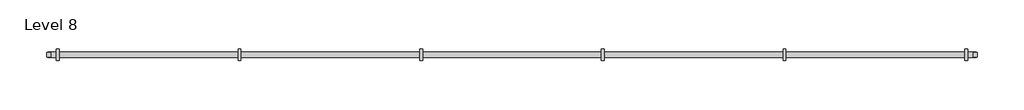
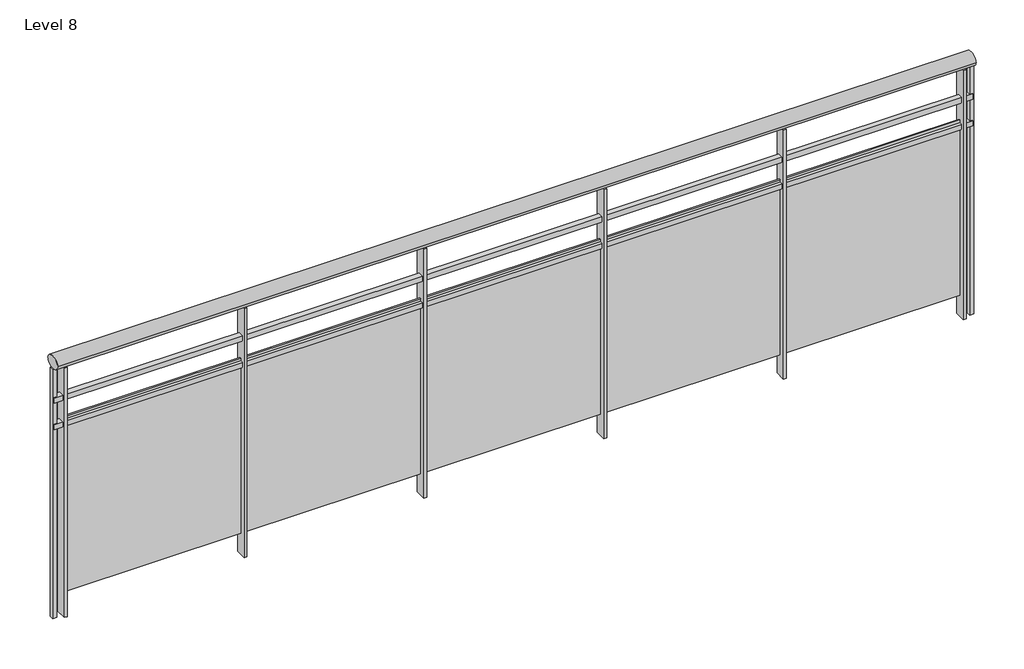
# One storey: 2 railings.
"""IFC4 building model written with IfcOpenShell, lengths in millimetres."""

from ifc_helpers import new_model, si_unit, point, frame, origin, place, context, project, spatial, polyline, ellipse_curve, trimmed, outline, extrude, element, save
from ifc_brep_helpers import plane_surface, extruded_surface, advanced_brep

model = new_model("IFC4")

# Units and contexts
model_context = context("Model", 3, world=origin())
ifc_project = project(units=[si_unit("LENGTHUNIT", "METRE", prefix="MILLI")], contexts=[model_context])

# Site, building, storey
site = spatial("IfcSite", under=ifc_project)
building = spatial("IfcBuilding", under=site)
storey = spatial("IfcBuildingStorey", under=building, Name="Level 8", Elevation=22402.8)

# Railings
placement = place(None, origin())
element("IfcRailing", 1, ObjectType="Glass Panel - Bottom Fill", at=placement, inside=storey, context=model_context, shape_type="SolidModel", body=[
    advanced_brep(
    [(-5729.1673724, -5829.5544725, 23622.0), (-5729.1673724, -5905.7544725, 23622.0), (-1576.8982041, -5829.5544725, 23622.0), (-1576.8982041, -5905.7544725, 23622.0)],
    [
        (0, 1, ellipse_curve(frame((-5729.1673724, -5867.6544725, 23622.0), z_axis=(-1.0, 0.0, 0.0), x_axis=(0.0, -1.0, 0.0)), 38.1, 28.575)),
        (1, 0, ellipse_curve(frame((-5729.1673724, -5867.6544725, 23622.0), z_axis=(-1.0, 0.0, 0.0), x_axis=(0.0, -1.0, 0.0)), 38.1, 28.575)),
        (2, 3, ellipse_curve(frame((-1576.8982041, -5867.6544725, 23622.0), z_axis=(1.0, 0.0, 0.0), x_axis=(0.0, -1.0, 0.0)), 38.1, 28.575)),
        (3, 2, ellipse_curve(frame((-1576.8982041, -5867.6544725, 23622.0), z_axis=(1.0, 0.0, 0.0), x_axis=(0.0, -1.0, 0.0)), 38.1, 28.575)),
        (0, 2),
        (3, 1),
    ],
    [
        plane_surface(frame((-5729.1673724, -5867.6544725, 23622.0), z_axis=(-1.0, 0.0, 0.0), x_axis=(0.0, 1.0, 0.0))),
        plane_surface(frame((-1576.8982041, -5867.6544725, 23622.0), z_axis=(1.0, 0.0, 0.0), x_axis=(0.0, 1.0, 0.0))),
        extruded_surface(trimmed(ellipse_curve(frame((-1576.8982041, -5867.6544725, 23622.0), z_axis=(-1.0, 0.0, 0.0), x_axis=(0.0, -1.0, 0.0)), 38.1, 28.575), [point((-1576.8982041, -5829.5544725, 23622.0))], [point((-1576.8982041, -5905.7544725, 23622.0))], True, "CARTESIAN"), (-4152.2691683, 0.0, 0.0), 4152.2691683),
        extruded_surface(trimmed(ellipse_curve(frame((-1576.8982041, -5867.6544725, 23622.0), z_axis=(-1.0, 0.0, 0.0), x_axis=(0.0, -1.0, 0.0)), 38.1, 28.575), [point((-1576.8982041, -5905.7544725, 23622.0))], [point((-1576.8982041, -5829.5544725, 23622.0))], True, "CARTESIAN"), (-4152.2691683, 0.0, 0.0), 4152.2691683),
    ],
    [
        (0, [[1, 2]]),
        (1, [[3, 4]]),
        (2, [[-1, 5, -4, 6]]),
        (3, [[-2, -6, -3, -5]]),
    ],
),
    extrude(outline(polyline([(-5729.1673724, -5880.3544725), (-5729.1673724, -5854.9544725), (-1576.8982041, -5854.9544725), (-1576.8982041, -5880.3544725), (-5729.1673724, -5880.3544725)])), frame((0.0, 0.0, 23431.5), z_axis=(0.0, 0.0, 1.0), x_axis=(1.0, 0.0, 0.0)), (0.0, 0.0, 1.0), 25.4),
    extrude(outline(polyline([(-5729.1673724, -5880.3544725), (-5729.1673724, -5854.9544725), (-1576.8982041, -5854.9544725), (-1576.8982041, -5880.3544725), (-5729.1673724, -5880.3544725)])), frame((0.0, 0.0, 23304.5), z_axis=(0.0, 0.0, 1.0), x_axis=(1.0, 0.0, 0.0)), (0.0, 0.0, 1.0), 25.4),
    extrude(outline(polyline([(-1627.3827882, -5893.0544725), (-1627.3827882, -5842.2544725), (-1614.6827882, -5842.2544725), (-1614.6827882, -5893.0544725), (-1627.3827882, -5893.0544725)])), frame((0.0, 0.0, 22402.8), z_axis=(0.0, 0.0, 1.0), x_axis=(1.0, 0.0, 0.0)), (0.0, 0.0, 1.0), 1190.625),
    extrude(outline(polyline([(-2433.8327882, -5861.1193155), (-1621.0327882, -5861.1193155), (-1621.0327882, -5867.4693155), (-2433.8327882, -5867.4693155), (-2433.8327882, -5861.1193155)])), frame((0.0, 0.0, 22504.4), z_axis=(0.0, 0.0, 1.0), x_axis=(1.0, 0.0, 0.0)), (0.0, 0.0, 1.0), 838.2),
    extrude(outline(polyline([(-2440.1827882, -5893.0544725), (-2440.1827882, -5842.2544725), (-2427.4827882, -5842.2544725), (-2427.4827882, -5893.0544725), (-2440.1827882, -5893.0544725)])), frame((0.0, 0.0, 22402.8), z_axis=(0.0, 0.0, 1.0), x_axis=(1.0, 0.0, 0.0)), (0.0, 0.0, 1.0), 1190.625),
    extrude(outline(polyline([(-3246.6327882, -5861.1193155), (-2433.8327882, -5861.1193155), (-2433.8327882, -5867.4693155), (-3246.6327882, -5867.4693155), (-3246.6327882, -5861.1193155)])), frame((0.0, 0.0, 22504.4), z_axis=(0.0, 0.0, 1.0), x_axis=(1.0, 0.0, 0.0)), (0.0, 0.0, 1.0), 838.2),
    extrude(outline(polyline([(-3252.9827882, -5893.0544725), (-3252.9827882, -5842.2544725), (-3240.2827882, -5842.2544725), (-3240.2827882, -5893.0544725), (-3252.9827882, -5893.0544725)])), frame((0.0, 0.0, 22402.8), z_axis=(0.0, 0.0, 1.0), x_axis=(1.0, 0.0, 0.0)), (0.0, 0.0, 1.0), 1190.625),
    extrude(outline(polyline([(-4059.4327882, -5861.1193155), (-3246.6327882, -5861.1193155), (-3246.6327882, -5867.4693155), (-4059.4327882, -5867.4693155), (-4059.4327882, -5861.1193155)])), frame((0.0, 0.0, 22504.4), z_axis=(0.0, 0.0, 1.0), x_axis=(1.0, 0.0, 0.0)), (0.0, 0.0, 1.0), 838.2),
    extrude(outline(polyline([(-4065.7827882, -5893.0544725), (-4065.7827882, -5842.2544725), (-4053.0827882, -5842.2544725), (-4053.0827882, -5893.0544725), (-4065.7827882, -5893.0544725)])), frame((0.0, 0.0, 22402.8), z_axis=(0.0, 0.0, 1.0), x_axis=(1.0, 0.0, 0.0)), (0.0, 0.0, 1.0), 1190.625),
    extrude(outline(polyline([(-4872.2327882, -5861.1193155), (-4059.4327882, -5861.1193155), (-4059.4327882, -5867.4693155), (-4872.2327882, -5867.4693155), (-4872.2327882, -5861.1193155)])), frame((0.0, 0.0, 22504.4), z_axis=(0.0, 0.0, 1.0), x_axis=(1.0, 0.0, 0.0)), (0.0, 0.0, 1.0), 838.2),
    extrude(outline(polyline([(-4878.5827882, -5893.0544725), (-4878.5827882, -5842.2544725), (-4865.8827882, -5842.2544725), (-4865.8827882, -5893.0544725), (-4878.5827882, -5893.0544725)])), frame((0.0, 0.0, 22402.8), z_axis=(0.0, 0.0, 1.0), x_axis=(1.0, 0.0, 0.0)), (0.0, 0.0, 1.0), 1190.625),
    extrude(outline(polyline([(-5685.0327882, -5861.1193155), (-4872.2327882, -5861.1193155), (-4872.2327882, -5867.4693155), (-5685.0327882, -5867.4693155), (-5685.0327882, -5861.1193155)])), frame((0.0, 0.0, 22504.4), z_axis=(0.0, 0.0, 1.0), x_axis=(1.0, 0.0, 0.0)), (0.0, 0.0, 1.0), 838.2),
    extrude(outline(polyline([(-5691.3827882, -5893.0544725), (-5691.3827882, -5842.2544725), (-5678.6827882, -5842.2544725), (-5678.6827882, -5893.0544725), (-5691.3827882, -5893.0544725)])), frame((0.0, 0.0, 22402.8), z_axis=(0.0, 0.0, 1.0), x_axis=(1.0, 0.0, 0.0)), (0.0, 0.0, 1.0), 1190.625),
    extrude(outline(polyline([(-1589.5982041, -5877.1794725), (-1589.5982041, -5858.1294725), (-1570.5482041, -5858.1294725), (-1570.5482041, -5877.1794725), (-1589.5982041, -5877.1794725)])), frame((0.0, 0.0, 22402.8), z_axis=(0.0, 0.0, 1.0), x_axis=(1.0, 0.0, 0.0)), (0.0, 0.0, 1.0), 1190.625),
    extrude(outline(polyline([(-5735.5173724, -5877.1794725), (-5735.5173724, -5858.1294725), (-5716.4673724, -5858.1294725), (-5716.4673724, -5877.1794725), (-5735.5173724, -5877.1794725)])), frame((0.0, 0.0, 22402.8), z_axis=(0.0, 0.0, 1.0), x_axis=(1.0, 0.0, 0.0)), (0.0, 0.0, 1.0), 1190.625),
])
element("IfcRailing", 2, ObjectType="Glass Panel - Bottom Fill", at=placement, inside=storey, context=model_context, shape_type="SolidModel", body=[
    advanced_brep(
    [(-5729.1673724, -5829.5544725, 23622.0), (-5729.1673724, -5905.7544725, 23622.0), (-1576.8982041, -5829.5544725, 23622.0), (-1576.8982041, -5905.7544725, 23622.0)],
    [
        (0, 1, ellipse_curve(frame((-5729.1673724, -5867.6544725, 23622.0), z_axis=(-1.0, 0.0, 0.0), x_axis=(0.0, -1.0, 0.0)), 38.1, 28.575)),
        (1, 0, ellipse_curve(frame((-5729.1673724, -5867.6544725, 23622.0), z_axis=(-1.0, 0.0, 0.0), x_axis=(0.0, -1.0, 0.0)), 38.1, 28.575)),
        (2, 3, ellipse_curve(frame((-1576.8982041, -5867.6544725, 23622.0), z_axis=(1.0, 0.0, 0.0), x_axis=(0.0, -1.0, 0.0)), 38.1, 28.575)),
        (3, 2, ellipse_curve(frame((-1576.8982041, -5867.6544725, 23622.0), z_axis=(1.0, 0.0, 0.0), x_axis=(0.0, -1.0, 0.0)), 38.1, 28.575)),
        (0, 2),
        (3, 1),
    ],
    [
        plane_surface(frame((-5729.1673724, -5867.6544725, 23622.0), z_axis=(-1.0, 0.0, 0.0), x_axis=(0.0, 1.0, 0.0))),
        plane_surface(frame((-1576.8982041, -5867.6544725, 23622.0), z_axis=(1.0, 0.0, 0.0), x_axis=(0.0, 1.0, 0.0))),
        extruded_surface(trimmed(ellipse_curve(frame((-1576.8982041, -5867.6544725, 23622.0), z_axis=(-1.0, 0.0, 0.0), x_axis=(0.0, -1.0, 0.0)), 38.1, 28.575), [point((-1576.8982041, -5829.5544725, 23622.0))], [point((-1576.8982041, -5905.7544725, 23622.0))], True, "CARTESIAN"), (-4152.2691683, 0.0, 0.0), 4152.2691683),
        extruded_surface(trimmed(ellipse_curve(frame((-1576.8982041, -5867.6544725, 23622.0), z_axis=(-1.0, 0.0, 0.0), x_axis=(0.0, -1.0, 0.0)), 38.1, 28.575), [point((-1576.8982041, -5905.7544725, 23622.0))], [point((-1576.8982041, -5829.5544725, 23622.0))], True, "CARTESIAN"), (-4152.2691683, 0.0, 0.0), 4152.2691683),
    ],
    [
        (0, [[1, 2]]),
        (1, [[3, 4]]),
        (2, [[-1, 5, -4, 6]]),
        (3, [[-2, -6, -3, -5]]),
    ],
),
    extrude(outline(polyline([(-5729.1673724, -5880.3544725), (-5729.1673724, -5854.9544725), (-1576.8982041, -5854.9544725), (-1576.8982041, -5880.3544725), (-5729.1673724, -5880.3544725)])), frame((0.0, 0.0, 23431.5), z_axis=(0.0, 0.0, 1.0), x_axis=(1.0, 0.0, 0.0)), (0.0, 0.0, 1.0), 25.4),
    extrude(outline(polyline([(-5729.1673724, -5880.3544725), (-5729.1673724, -5854.9544725), (-1576.8982041, -5854.9544725), (-1576.8982041, -5880.3544725), (-5729.1673724, -5880.3544725)])), frame((0.0, 0.0, 23304.5), z_axis=(0.0, 0.0, 1.0), x_axis=(1.0, 0.0, 0.0)), (0.0, 0.0, 1.0), 25.4),
    extrude(outline(polyline([(-1627.3827882, -5893.0544725), (-1627.3827882, -5842.2544725), (-1614.6827882, -5842.2544725), (-1614.6827882, -5893.0544725), (-1627.3827882, -5893.0544725)])), frame((0.0, 0.0, 22402.8), z_axis=(0.0, 0.0, 1.0), x_axis=(1.0, 0.0, 0.0)), (0.0, 0.0, 1.0), 1190.625),
    extrude(outline(polyline([(-2433.8327882, -5861.1193155), (-1621.0327882, -5861.1193155), (-1621.0327882, -5867.4693155), (-2433.8327882, -5867.4693155), (-2433.8327882, -5861.1193155)])), frame((0.0, 0.0, 22504.4), z_axis=(0.0, 0.0, 1.0), x_axis=(1.0, 0.0, 0.0)), (0.0, 0.0, 1.0), 838.2),
    extrude(outline(polyline([(-2440.1827882, -5893.0544725), (-2440.1827882, -5842.2544725), (-2427.4827882, -5842.2544725), (-2427.4827882, -5893.0544725), (-2440.1827882, -5893.0544725)])), frame((0.0, 0.0, 22402.8), z_axis=(0.0, 0.0, 1.0), x_axis=(1.0, 0.0, 0.0)), (0.0, 0.0, 1.0), 1190.625),
    extrude(outline(polyline([(-3246.6327882, -5861.1193155), (-2433.8327882, -5861.1193155), (-2433.8327882, -5867.4693155), (-3246.6327882, -5867.4693155), (-3246.6327882, -5861.1193155)])), frame((0.0, 0.0, 22504.4), z_axis=(0.0, 0.0, 1.0), x_axis=(1.0, 0.0, 0.0)), (0.0, 0.0, 1.0), 838.2),
    extrude(outline(polyline([(-3252.9827882, -5893.0544725), (-3252.9827882, -5842.2544725), (-3240.2827882, -5842.2544725), (-3240.2827882, -5893.0544725), (-3252.9827882, -5893.0544725)])), frame((0.0, 0.0, 22402.8), z_axis=(0.0, 0.0, 1.0), x_axis=(1.0, 0.0, 0.0)), (0.0, 0.0, 1.0), 1190.625),
    extrude(outline(polyline([(-4059.4327882, -5861.1193155), (-3246.6327882, -5861.1193155), (-3246.6327882, -5867.4693155), (-4059.4327882, -5867.4693155), (-4059.4327882, -5861.1193155)])), frame((0.0, 0.0, 22504.4), z_axis=(0.0, 0.0, 1.0), x_axis=(1.0, 0.0, 0.0)), (0.0, 0.0, 1.0), 838.2),
    extrude(outline(polyline([(-4065.7827882, -5893.0544725), (-4065.7827882, -5842.2544725), (-4053.0827882, -5842.2544725), (-4053.0827882, -5893.0544725), (-4065.7827882, -5893.0544725)])), frame((0.0, 0.0, 22402.8), z_axis=(0.0, 0.0, 1.0), x_axis=(1.0, 0.0, 0.0)), (0.0, 0.0, 1.0), 1190.625),
    extrude(outline(polyline([(-4872.2327882, -5861.1193155), (-4059.4327882, -5861.1193155), (-4059.4327882, -5867.4693155), (-4872.2327882, -5867.4693155), (-4872.2327882, -5861.1193155)])), frame((0.0, 0.0, 22504.4), z_axis=(0.0, 0.0, 1.0), x_axis=(1.0, 0.0, 0.0)), (0.0, 0.0, 1.0), 838.2),
    extrude(outline(polyline([(-4878.5827882, -5893.0544725), (-4878.5827882, -5842.2544725), (-4865.8827882, -5842.2544725), (-4865.8827882, -5893.0544725), (-4878.5827882, -5893.0544725)])), frame((0.0, 0.0, 22402.8), z_axis=(0.0, 0.0, 1.0), x_axis=(1.0, 0.0, 0.0)), (0.0, 0.0, 1.0), 1190.625),
    extrude(outline(polyline([(-5685.0327882, -5861.1193155), (-4872.2327882, -5861.1193155), (-4872.2327882, -5867.4693155), (-5685.0327882, -5867.4693155), (-5685.0327882, -5861.1193155)])), frame((0.0, 0.0, 22504.4), z_axis=(0.0, 0.0, 1.0), x_axis=(1.0, 0.0, 0.0)), (0.0, 0.0, 1.0), 838.2),
    extrude(outline(polyline([(-5691.3827882, -5893.0544725), (-5691.3827882, -5842.2544725), (-5678.6827882, -5842.2544725), (-5678.6827882, -5893.0544725), (-5691.3827882, -5893.0544725)])), frame((0.0, 0.0, 22402.8), z_axis=(0.0, 0.0, 1.0), x_axis=(1.0, 0.0, 0.0)), (0.0, 0.0, 1.0), 1190.625),
    extrude(outline(polyline([(-1589.5982041, -5877.1794725), (-1589.5982041, -5858.1294725), (-1570.5482041, -5858.1294725), (-1570.5482041, -5877.1794725), (-1589.5982041, -5877.1794725)])), frame((0.0, 0.0, 22402.8), z_axis=(0.0, 0.0, 1.0), x_axis=(1.0, 0.0, 0.0)), (0.0, 0.0, 1.0), 1190.625),
    extrude(outline(polyline([(-5735.5173724, -5877.1794725), (-5735.5173724, -5858.1294725), (-5716.4673724, -5858.1294725), (-5716.4673724, -5877.1794725), (-5735.5173724, -5877.1794725)])), frame((0.0, 0.0, 22402.8), z_axis=(0.0, 0.0, 1.0), x_axis=(1.0, 0.0, 0.0)), (0.0, 0.0, 1.0), 1190.625),
])

save(model, "model.ifc")

# Revit data of these elements
# Type "Glass Panel - Bottom Fill"
#   Assembly Code = "C2010400"
#   built-in parameter 1008612 = 0.0416667 (stored number, unit not read)
#   built-in parameter 1008611 = 0.0416667 (stored number, unit not read)
#   built-in parameter 1008609 = 0.333333 (stored number, unit not read)
#   built-in parameter 1008604 = 0.166667 (stored number, unit not read)
#   built-in parameter 1008603 = 0.166667 (stored number, unit not read)
#   Railing Height = 4' - 0"
#   built-in parameter 1008630 = 2
#   built-in parameter 1008610 = 2
#   built-in parameter 1008618 = Baluster - Square : 3/4"
# Elements 1, 2 (IfcRailing, "Glass Panel - Bottom Fill")
#   Phase Created = New Construction
#   Materials on its faces: "Glass"
# Materials
#   "Glass": class "Glass", colour RGB 0 128 192, transparency 0.75, Description = "Soda Lime Glass", Cost = 0
